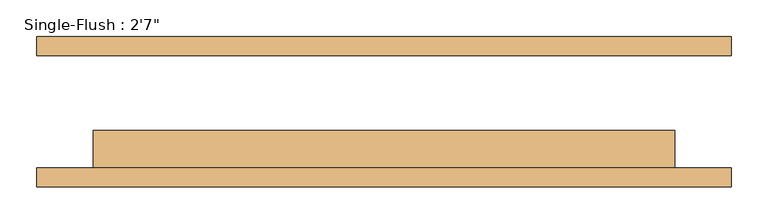
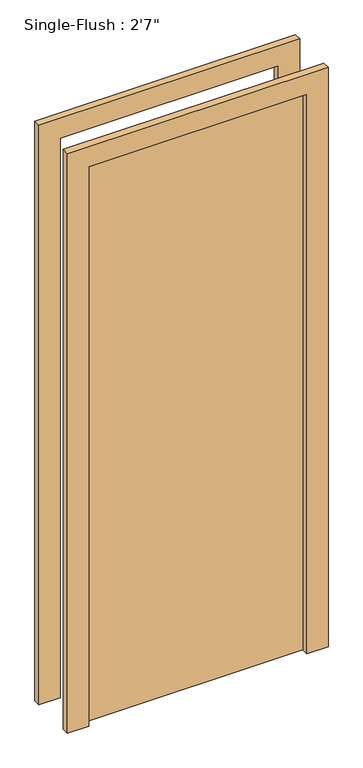
"""IFC4 building model written with IfcOpenShell, lengths in millimetres: door geometry."""

from ifc_helpers import new_model, si_unit, frame, origin, origin_with_axes, place, context, project, spatial, polyline, outline, extrude, source, transform, mapped, element, save


def door_dc34e247(model_context):
    return source(origin(), model_context, "Body", "SweptSolid", [
        extrude(outline(polyline([(2209.8, -469.9), (0.0, -469.9), (0.0, -393.7), (2133.6, -393.7), (2133.6, 393.7), (0.0, 393.7), (0.0, 469.9), (2209.8, 469.9), (2209.8, -469.9)])), frame((0.0, -101.6, 0.0), z_axis=(0.0, 1.0, 0.0), x_axis=(0.0, 0.0, 1.0)), (0.0, 0.0, 1.0), 25.4),
        extrude(outline(polyline([(2209.8, 469.9), (2209.8, -469.9), (0.0, -469.9), (0.0, -393.7), (2133.6, -393.7), (2133.6, 393.7), (0.0, 393.7), (0.0, 469.9), (2209.8, 469.9)])), frame((0.0, 76.2, 0.0), z_axis=(0.0, 1.0, 0.0), x_axis=(0.0, 0.0, 1.0)), (0.0, 0.0, 1.0), 25.4),
        extrude(outline(polyline([(393.7, -25.4), (393.7, -76.2), (-393.7, -76.2), (-393.7, -25.4), (393.7, -25.4)])), origin_with_axes(), (0.0, 0.0, 1.0), 2133.6),
    ])


if __name__ == "__main__":
    model = new_model("IFC4")
    model_context = context("Model", 3, world=origin())
    ifc_project = project(units=[si_unit("LENGTHUNIT", "METRE", prefix="MILLI")], contexts=[model_context])
    site = spatial("IfcSite", under=ifc_project)
    building = spatial("IfcBuilding", under=site)
    placement = place(None, origin())
    door_shape = door_dc34e247(model_context)
    element("IfcDoor", 1, ObjectType="Single-Flush : 2'7\"", at=placement, inside=building, context=model_context, shape_type="MappedRepresentation", body=[
        mapped(door_shape, transform((0.0, 0.0, 0.0), x_axis=(1.0, 0.0, 0.0), y_axis=(0.0, 1.0, 0.0), z_axis=(0.0, 0.0, 1.0))),
    ])
    save(model, "model.ifc")

# Revit data of these elements
# Type "Single-Flush : 2'7\""
#   Type Mark = "8"
#   Construction Type Id = "MDOOR"
#   Assembly Code = "C1020"
#   Analytic Construction = "Metal"
#   Thickness = 0' - 2"
#   Heat Transfer Coefficient (U) = 0.651978 BTU/(h·ft²·°F)
#   Height = 7' - 0"
#   Trim Projection Ext = 0' - 1"
#   Trim Projection Int = 0' - 1"
#   Trim Width = 0' - 3"
#   Width = 2' - 7"
#   Define Thermal Properties by = 1
#   Door Material = Door - Panel
#   Frame Material = Door - Frame
#   Visual Light Transmittance = 0
#   Solar Heat Gain Coefficient = 0
#   Function = (empty or 0)
#   Wall Closure = (empty or 0)
# Element 1 (IfcDoor, "Single-Flush : 2'7\"")
#   Materials on its faces: "Door - Frame", "Door - Panel"
# Materials
#   "Door - Panel": class "Wood", colour RGB 210 159 95, transparency 0
#   "Door - Frame": colour RGB 118 70 51, transparency 0
